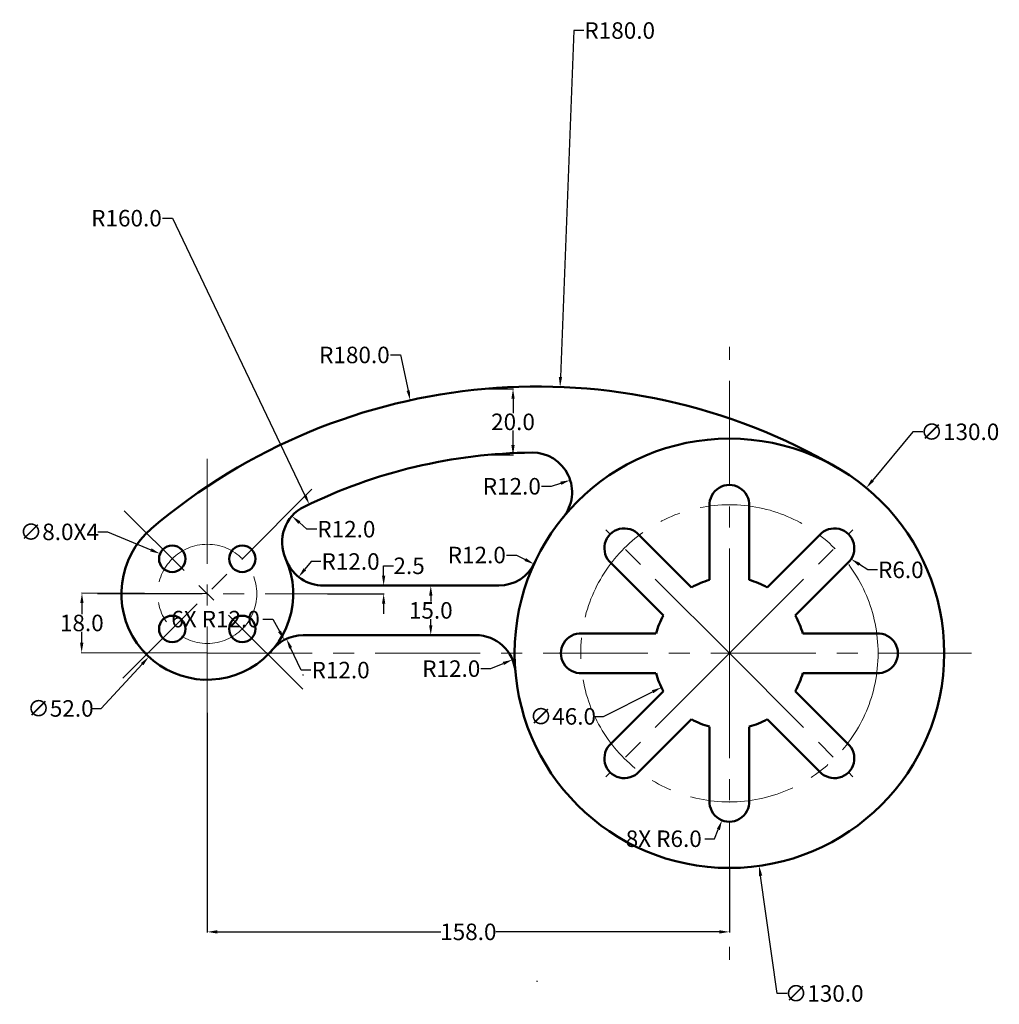
# Model space of a CAD drawing. Units: inches. Extents: x 143 to 440, y 43 to 341.
import ezdxf

# ---------------------------------------------------------------- set-up
doc = ezdxf.new("R2010")
doc.units = ezdxf.units.IN
doc.header["$MEASUREMENT"] = 0
doc.linetypes.add('CENTER', pattern=[50.8, 31.75, -6.35, 6.35, -6.35])
for name, color, linetype, lineweight in [('M-CNTR', 4, 'CENTER', 18), ('M-DIMS', 2, 'Continuous', 25), ('M-OUTL', 7, 'Continuous', 50)]:
    doc.layers.add(name, color=color, linetype=linetype, lineweight=lineweight)
doc.styles.get("Standard").update_dxf_attribs({"font": 'arial.ttf'})
doc.dimstyles.get("Standard").update_dxf_attribs({"dimtxt": 5, "dimasz": 3, "dimexe": 0.18, "dimexo": 0.0625, "dimgap": 0.09, "dimtad": 0, "dimtih": 1, "dimtoh": 1, "dimdec": 1, "dimzin": 0, "dimdsep": 46, "dimtxsty": 'Standard', "dimcen": 0.09, "dimadec": 0, "dimazin": 0, "dimtfac": 1, "dimtdec": 1, "dimtofl": 0, "dimtmove": 0, "dimatfit": 3, "dimfxl": 1, "dimtolj": 1, "dimtzin": 0, "dimarcsym": 0})

# ---------------------------------------------------------------- blocks, each defined once
blk = doc.blocks.new('*D1')
at = {"layer": 'Defpoints', "color": 0, "transparency": 16777216}
for p in [(217.9, 186.39), (182.55, 148.25)]:
    blk.add_point(p, dxfattribs=at)
at = {"layer": 'M-DIMS', "color": 0, "lineweight": -2, "transparency": 16777216}
for p, q in [((200.14, 167.32), (200.32, 167.32)), ((200.23, 167.23), (200.23, 167.41)), ((168.09, 132.63), (180.52, 146.05)), ((165.09, 132.63), (168.09, 132.63))]:
    blk.add_line(p, q, dxfattribs=at)
at = {"layer": 'M-DIMS', "color": 0, "transparency": 16777216}
blk.add_solid([(180.15, 146.39), (180.88, 145.71), (182.55, 148.25)], dxfattribs=at)
at = {"layer": 'M-DIMS', "color": 0, "transparency": 16777216, "insert": (155.79, 132.63), "char_height": 5, "attachment_point": 5}
blk.add_mtext('\\A1;∅52.0', dxfattribs=at)
blk = doc.blocks.new('*D2')
at = {"layer": 'Defpoints', "color": 0, "transparency": 16777216}
for p in [(399.68, 199.38), (316.77, 99.26)]:
    blk.add_point(p, dxfattribs=at)
at = {"layer": 'M-DIMS', "color": 0, "lineweight": -2, "transparency": 16777216}
for p, q in [((413.75, 216.38), (401.59, 201.69)), ((416.75, 216.38), (413.75, 216.38)), ((358.14, 149.32), (358.32, 149.32)), ((358.23, 149.23), (358.23, 149.41))]:
    blk.add_line(p, q, dxfattribs=at)
at = {"layer": 'M-DIMS', "color": 0, "transparency": 16777216}
blk.add_solid([(401.21, 202.01), (401.98, 201.38), (399.68, 199.38)], dxfattribs=at)
at = {"layer": 'M-DIMS', "color": 0, "transparency": 16777216, "insert": (427.99, 216.38), "char_height": 5, "attachment_point": 5}
blk.add_mtext('\\A1;∅130.0', dxfattribs=at)
blk = doc.blocks.new('*D3')
at = {"layer": 'Defpoints', "color": 0, "transparency": 16777216}
for p in [(236.57, 167.32), (243.16, 169.82), (253.6, 169.82)]:
    blk.add_point(p, dxfattribs=at)
at = {"layer": 'M-DIMS', "color": 0, "lineweight": -2, "transparency": 16777216}
for p, q in [((253.6, 172.82), (253.6, 175.82)), ((253.6, 175.82), (256.6, 175.82)), ((236.63, 167.32), (253.78, 167.32)), ((243.22, 169.82), (253.78, 169.82)), ((253.6, 164.32), (253.6, 161.32))]:
    blk.add_line(p, q, dxfattribs=at)
at = {"layer": 'M-DIMS', "color": 0, "transparency": 16777216}
for points in [[(253.1, 172.82), (254.1, 172.82), (253.6, 169.82)], [(253.1, 164.32), (254.1, 164.32), (253.6, 167.32)]]:
    blk.add_solid(points, dxfattribs=at)
at = {"layer": 'M-DIMS', "color": 0, "transparency": 16777216, "insert": (261.3, 175.82), "char_height": 5, "attachment_point": 5}
blk.add_mtext('\\A1;2.5', dxfattribs=at)
blk = doc.blocks.new('*D4')
at = {"layer": 'Defpoints', "color": 0, "transparency": 16777216}
for p in [(267.86, 169.82), (263.59, 154.82), (267.86, 154.82)]:
    blk.add_point(p, dxfattribs=at)
at = {"layer": 'M-DIMS', "color": 0, "lineweight": -2, "transparency": 16777216}
for p, q in [((267.92, 169.82), (268.04, 169.82)), ((267.86, 166.82), (267.86, 164.96)), ((267.86, 157.82), (267.86, 159.68)), ((263.65, 154.82), (268.04, 154.82))]:
    blk.add_line(p, q, dxfattribs=at)
at = {"layer": 'M-DIMS', "color": 0, "transparency": 16777216}
for points in [[(267.36, 166.82), (268.36, 166.82), (267.86, 169.82)], [(267.36, 157.82), (268.36, 157.82), (267.86, 154.82)]]:
    blk.add_solid(points, dxfattribs=at)
at = {"layer": 'M-DIMS', "color": 0, "transparency": 16777216, "insert": (267.86, 162.32), "char_height": 5, "attachment_point": 5}
blk.add_mtext('\\A1;15.0', dxfattribs=at)
blk = doc.blocks.new('*D5')
at = {"layer": 'Defpoints', "color": 0, "transparency": 16777216}
for p in [(261.65, 225.94), (300.09, 50.09)]:
    blk.add_point(p, dxfattribs=at)
at = {"layer": 'M-DIMS', "color": 0, "lineweight": -2, "transparency": 16777216}
for p, q in [((255.66, 239.66), (258.66, 239.66)), ((258.66, 239.66), (261.01, 228.87)), ((300, 50.09), (300.18, 50.09)), ((300.09, 50), (300.09, 50.18))]:
    blk.add_line(p, q, dxfattribs=at)
at = {"layer": 'M-DIMS', "color": 0, "transparency": 16777216}
blk.add_solid([(261.5, 228.98), (260.53, 228.77), (261.65, 225.94)], dxfattribs=at)
at = {"layer": 'M-DIMS', "color": 0, "transparency": 16777216, "insert": (244.75, 239.66), "char_height": 5, "attachment_point": 5}
blk.add_mtext('\\A1;R180.0', dxfattribs=at)
blk = doc.blocks.new('*U6')
blk.add_circle((0, 0), 4)
blk = doc.blocks.new('*U7')
at = {"layer": 'M-OUTL', "color": 0, "linetype": 'ByBlock', "lineweight": -2, "transparency": 16777216}
for p, rotation in [((189.62, 177.93), 89.99999999999999), ((189.62, 156.71), 180), ((210.83, 156.71), 270)]:
    blk.add_blockref('*U6', p, dxfattribs=dict(at, rotation=rotation))
blk.add_blockref('*U6', (210.83, 177.93), dxfattribs=at)
blk = doc.blocks.new('*D8')
at = {"layer": 'Defpoints', "color": 0, "transparency": 16777216}
for p in [(185.93, 179.47), (193.31, 176.39)]:
    blk.add_point(p, dxfattribs=at)
at = {"layer": 'M-DIMS', "color": 0, "lineweight": -2, "transparency": 16777216}
for p, q in [((167.07, 186.09), (170.07, 186.09)), ((170.07, 186.09), (183.16, 180.62)), ((189.53, 177.93), (189.71, 177.93)), ((189.62, 177.84), (189.62, 178.02))]:
    blk.add_line(p, q, dxfattribs=at)
at = {"layer": 'M-DIMS', "color": 0, "transparency": 16777216}
blk.add_solid([(183.35, 181.09), (182.97, 180.16), (185.93, 179.47)], dxfattribs=at)
at = {"layer": 'M-DIMS', "color": 0, "transparency": 16777216, "insert": (155.45, 186.09), "char_height": 5, "attachment_point": 5}
blk.add_mtext('\\A1;∅8.0X4', dxfattribs=at)
blk = doc.blocks.new('*D9')
at = {"layer": 'Defpoints', "color": 0, "transparency": 16777216}
for p in [(224.19, 153.69), (229.27, 142.82)]:
    blk.add_point(p, dxfattribs=at)
at = {"layer": 'M-DIMS', "color": 0, "lineweight": -2, "transparency": 16777216}
for p, q in [((228.61, 144.24), (225.46, 150.97)), ((231.61, 144.24), (228.61, 144.24))]:
    blk.add_line(p, q, dxfattribs=at)
at = {"layer": 'M-DIMS', "color": 0, "transparency": 16777216}
blk.add_solid([(225.91, 151.18), (225, 150.76), (224.19, 153.69)], dxfattribs=at)
at = {"layer": 'M-DIMS', "color": 0, "transparency": 16777216, "insert": (240.58, 144.24), "char_height": 5, "attachment_point": 5}
blk.add_mtext('\\A1;R12.0', dxfattribs=at)
blk = doc.blocks.new('*D10')
at = {"layer": 'Defpoints', "color": 0, "transparency": 16777216}
for p in [(292.6, 147.39), (281.5, 142.82)]:
    blk.add_point(p, dxfattribs=at)
at = {"layer": 'M-DIMS', "color": 0, "lineweight": -2, "transparency": 16777216}
for p, q in [((286.03, 144.68), (289.82, 146.24)), ((283.03, 144.68), (286.03, 144.68))]:
    blk.add_line(p, q, dxfattribs=at)
at = {"layer": 'M-DIMS', "color": 0, "transparency": 16777216}
blk.add_solid([(289.63, 146.71), (290.01, 145.78), (292.6, 147.39)], dxfattribs=at)
at = {"layer": 'M-DIMS', "color": 0, "transparency": 16777216, "insert": (274.06, 144.68), "char_height": 5, "attachment_point": 5}
blk.add_mtext('\\A1;R12.0', dxfattribs=at)
blk = doc.blocks.new('*D11')
at = {"layer": 'Defpoints', "color": 0, "transparency": 16777216}
for p in [(225.85, 190.86), (234.86, 182.94)]:
    blk.add_point(p, dxfattribs=at)
at = {"layer": 'M-DIMS', "color": 0, "lineweight": -2, "transparency": 16777216}
for p, q in [((230.36, 186.9), (228.1, 188.88)), ((233.36, 186.9), (230.36, 186.9))]:
    blk.add_line(p, q, dxfattribs=at)
at = {"layer": 'M-DIMS', "color": 0, "transparency": 16777216}
blk.add_solid([(228.43, 189.26), (227.77, 188.51), (225.85, 190.86)], dxfattribs=at)
at = {"layer": 'M-DIMS', "color": 0, "transparency": 16777216, "insert": (242.32, 186.9), "char_height": 5, "attachment_point": 5}
blk.add_mtext('\\A1;R12.0', dxfattribs=at)
blk = doc.blocks.new('*D12')
at = {"layer": 'Defpoints', "color": 0, "transparency": 16777216}
for p in [(235.35, 181.82), (227.89, 172.42)]:
    blk.add_point(p, dxfattribs=at)
at = {"layer": 'M-DIMS', "color": 0, "lineweight": -2, "transparency": 16777216}
for p, q in [((231.62, 177.12), (229.76, 174.77)), ((234.62, 177.12), (231.62, 177.12))]:
    blk.add_line(p, q, dxfattribs=at)
at = {"layer": 'M-DIMS', "color": 0, "transparency": 16777216}
blk.add_solid([(229.36, 175.08), (230.15, 174.46), (227.89, 172.42)], dxfattribs=at)
at = {"layer": 'M-DIMS', "color": 0, "transparency": 16777216, "insert": (243.59, 177.12), "char_height": 5, "attachment_point": 5}
blk.add_mtext('\\A1;R12.0', dxfattribs=at)
blk = doc.blocks.new('*D13')
at = {"layer": 'Defpoints', "color": 0, "transparency": 16777216}
for p in [(288.42, 181.82), (299.1, 176.34)]:
    blk.add_point(p, dxfattribs=at)
at = {"layer": 'M-DIMS', "color": 0, "lineweight": -2, "transparency": 16777216}
for p, q in [((290.76, 179.08), (293.76, 179.08)), ((293.76, 179.08), (296.43, 177.71))]:
    blk.add_line(p, q, dxfattribs=at)
at = {"layer": 'M-DIMS', "color": 0, "transparency": 16777216}
blk.add_solid([(296.66, 178.16), (296.2, 177.27), (299.1, 176.34)], dxfattribs=at)
at = {"layer": 'M-DIMS', "color": 0, "transparency": 16777216, "insert": (281.79, 179.08), "char_height": 5, "attachment_point": 5}
blk.add_mtext('\\A1;R12.0', dxfattribs=at)
blk = doc.blocks.new('*D14')
at = {"layer": 'Defpoints', "color": 0, "transparency": 16777216}
for p in [(310.07, 201.72), (298.64, 198.09)]:
    blk.add_point(p, dxfattribs=at)
at = {"layer": 'M-DIMS', "color": 0, "lineweight": -2, "transparency": 16777216}
for p, q in [((301.35, 199.9), (304.35, 199.9)), ((304.35, 199.9), (307.21, 200.81))]:
    blk.add_line(p, q, dxfattribs=at)
at = {"layer": 'M-DIMS', "color": 0, "transparency": 16777216}
blk.add_solid([(307.06, 201.29), (307.36, 200.34), (310.07, 201.72)], dxfattribs=at)
at = {"layer": 'M-DIMS', "color": 0, "transparency": 16777216, "insert": (292.39, 199.9), "char_height": 5, "attachment_point": 5}
blk.add_mtext('\\A1;R12.0', dxfattribs=at)
blk = doc.blocks.new('*D15')
at = {"layer": 'Defpoints', "color": 0, "transparency": 16777216}
for p in [(284.3, 229.4), (284.3, 209.4), (292.75, 209.4)]:
    blk.add_point(p, dxfattribs=at)
at = {"layer": 'M-DIMS', "color": 0, "lineweight": -2, "transparency": 16777216}
for p, q in [((284.37, 229.4), (292.93, 229.4)), ((292.75, 226.4), (292.75, 222.04)), ((292.75, 212.4), (292.75, 216.76)), ((284.37, 209.4), (292.93, 209.4))]:
    blk.add_line(p, q, dxfattribs=at)
at = {"layer": 'M-DIMS', "color": 0, "transparency": 16777216}
for points in [[(292.25, 226.4), (293.25, 226.4), (292.75, 229.4)], [(292.25, 212.4), (293.25, 212.4), (292.75, 209.4)]]:
    blk.add_solid(points, dxfattribs=at)
at = {"layer": 'M-DIMS', "color": 0, "transparency": 16777216, "insert": (292.75, 219.4), "char_height": 5, "attachment_point": 5}
blk.add_mtext('\\A1;20.0', dxfattribs=at)
blk = doc.blocks.new('*D16')
at = {"layer": 'Defpoints', "color": 0, "transparency": 16777216}
for p in [(200.32, 167.32), (162.21, 149.51), (200.23, 149.32)]:
    blk.add_point(p, dxfattribs=at)
at = {"layer": 'M-DIMS', "color": 0, "lineweight": -2, "transparency": 16777216}
for p, q in [((200.25, 167.32), (162.12, 167.51)), ((162.28, 164.51), (162.27, 161.15)), ((162.22, 152.51), (162.24, 155.87)), ((200.16, 149.32), (162.03, 149.51))]:
    blk.add_line(p, q, dxfattribs=at)
at = {"layer": 'M-DIMS', "color": 0, "transparency": 16777216}
for points in [[(161.78, 164.51), (162.78, 164.51), (162.3, 167.51)], [(161.72, 152.51), (162.72, 152.51), (162.21, 149.51)]]:
    blk.add_solid(points, dxfattribs=at)
at = {"layer": 'M-DIMS', "color": 0, "transparency": 16777216, "insert": (162.25, 158.51), "char_height": 5, "attachment_point": 5}
blk.add_mtext('\\A1;18.0', dxfattribs=at)
blk = doc.blocks.new('*D17')
at = {"layer": 'Defpoints', "color": 0, "transparency": 16777216}
for p in [(390.04, 181.14), (395.07, 177.87)]:
    blk.add_point(p, dxfattribs=at)
at = {"layer": 'M-DIMS', "color": 0, "lineweight": -2, "transparency": 16777216}
for p, q in [((389.95, 181.14), (390.13, 181.14)), ((390.04, 181.05), (390.04, 181.23)), ((400.1, 174.59), (397.59, 176.23)), ((403.1, 174.59), (400.1, 174.59))]:
    blk.add_line(p, q, dxfattribs=at)
at = {"layer": 'M-DIMS', "color": 0, "transparency": 16777216}
blk.add_solid([(397.86, 176.65), (397.32, 175.81), (395.07, 177.87)], dxfattribs=at)
at = {"layer": 'M-DIMS', "color": 0, "transparency": 16777216, "insert": (410.13, 174.59), "char_height": 5, "attachment_point": 5}
blk.add_mtext('\\A1;R6.0', dxfattribs=at)
blk = doc.blocks.new('*D18')
at = {"layer": 'Defpoints', "color": 0, "transparency": 16777216}
for p in [(378.78, 159.63), (337.67, 139.01)]:
    blk.add_point(p, dxfattribs=at)
at = {"layer": 'M-DIMS', "color": 0, "lineweight": -2, "transparency": 16777216}
for p, q in [((358.14, 149.32), (358.32, 149.32)), ((358.23, 149.23), (358.23, 149.41)), ((320.13, 130.22), (334.98, 137.66)), ((317.13, 130.22), (320.13, 130.22))]:
    blk.add_line(p, q, dxfattribs=at)
at = {"layer": 'M-DIMS', "color": 0, "transparency": 16777216}
blk.add_solid([(334.76, 138.11), (335.21, 137.22), (337.67, 139.01)], dxfattribs=at)
at = {"layer": 'M-DIMS', "color": 0, "transparency": 16777216, "insert": (307.83, 130.22), "char_height": 5, "attachment_point": 5}
blk.add_mtext('\\A1;∅46.0', dxfattribs=at)
blk = doc.blocks.new('*D19')
at = {"layer": 'Defpoints', "color": 0, "transparency": 16777216}
for p in [(200.23, 131.31), (358.23, 84.32), (200.23, 64.98)]:
    blk.add_point(p, dxfattribs=at)
at = {"layer": 'M-DIMS', "color": 0, "lineweight": -2, "transparency": 16777216}
for p, q in [((200.23, 131.25), (200.23, 64.8)), ((358.23, 84.26), (358.23, 64.8)), ((203.23, 64.98), (270.94, 64.98)), ((355.23, 64.98), (287.51, 64.98))]:
    blk.add_line(p, q, dxfattribs=at)
at = {"layer": 'M-DIMS', "color": 0, "transparency": 16777216}
for points in [[(203.23, 65.48), (203.23, 64.48), (200.23, 64.98)], [(355.23, 65.48), (355.23, 64.48), (358.23, 64.98)]]:
    blk.add_solid(points, dxfattribs=at)
at = {"layer": 'M-DIMS', "color": 0, "transparency": 16777216, "insert": (279.23, 64.98), "char_height": 5, "attachment_point": 5}
blk.add_mtext('\\A1;158.0', dxfattribs=at)
blk = doc.blocks.new('*D20')
at = {"layer": 'Defpoints', "color": 0, "transparency": 16777216}
for p in [(307, 229.96), (300.09, 50.09)]:
    blk.add_point(p, dxfattribs=at)
at = {"layer": 'M-DIMS', "color": 0, "lineweight": -2, "transparency": 16777216}
for p, q in [((311.14, 337.88), (307.11, 232.96)), ((314.14, 337.88), (311.14, 337.88)), ((300, 50.09), (300.18, 50.09)), ((300.09, 50), (300.09, 50.18))]:
    blk.add_line(p, q, dxfattribs=at)
at = {"layer": 'M-DIMS', "color": 0, "transparency": 16777216}
blk.add_solid([(306.61, 232.98), (307.61, 232.94), (307, 229.96)], dxfattribs=at)
at = {"layer": 'M-DIMS', "color": 0, "transparency": 16777216, "insert": (325.05, 337.88), "char_height": 5, "attachment_point": 5}
blk.add_mtext('\\A1;R180.0', dxfattribs=at)
blk = doc.blocks.new('*D21')
at = {"layer": 'Defpoints', "color": 0, "transparency": 16777216}
for p in [(231.09, 194.45), (300.09, 50.09)]:
    blk.add_point(p, dxfattribs=at)
at = {"layer": 'M-DIMS', "color": 0, "lineweight": -2, "transparency": 16777216}
for p, q in [((186.68, 281.06), (189.68, 281.06)), ((189.68, 281.06), (229.79, 197.15)), ((300, 50.09), (300.18, 50.09)), ((300.09, 50), (300.09, 50.18))]:
    blk.add_line(p, q, dxfattribs=at)
at = {"layer": 'M-DIMS', "color": 0, "transparency": 16777216}
blk.add_solid([(230.24, 197.37), (229.34, 196.94), (231.09, 194.45)], dxfattribs=at)
at = {"layer": 'M-DIMS', "color": 0, "transparency": 16777216, "insert": (175.77, 281.06), "char_height": 5, "attachment_point": 5}
blk.add_mtext('\\A1;R160.0', dxfattribs=at)
blk = doc.blocks.new('*D22')
at = {"layer": 'Defpoints', "color": 0, "transparency": 16777216}
for p in [(223.53, 153.36), (229.27, 142.82)]:
    blk.add_point(p, dxfattribs=at)
at = {"layer": 'M-DIMS', "color": 0, "lineweight": -2, "transparency": 16777216}
for p, q in [((217.08, 159.68), (220.08, 159.68)), ((220.08, 159.68), (222.09, 155.99)), ((229.18, 142.82), (229.36, 142.82)), ((229.27, 142.73), (229.27, 142.91))]:
    blk.add_line(p, q, dxfattribs=at)
at = {"layer": 'M-DIMS', "color": 0, "transparency": 16777216}
blk.add_solid([(222.53, 156.23), (221.65, 155.75), (223.53, 153.36)], dxfattribs=at)
at = {"layer": 'M-DIMS', "color": 0, "transparency": 16777216, "insert": (202.73, 159.68), "char_height": 5, "attachment_point": 5}
blk.add_mtext('\\A1;6X R12.0', dxfattribs=at)
blk = doc.blocks.new('*D23')
at = {"layer": 'Defpoints', "color": 0, "transparency": 16777216}
for p in [(349.19, 213.69), (367.26, 84.95)]:
    blk.add_point(p, dxfattribs=at)
at = {"layer": 'M-DIMS', "color": 0, "lineweight": -2, "transparency": 16777216}
for p, q in [((358.14, 149.32), (358.32, 149.32)), ((358.23, 149.23), (358.23, 149.41)), ((372.68, 46.33), (367.68, 81.98)), ((375.68, 46.33), (372.68, 46.33))]:
    blk.add_line(p, q, dxfattribs=at)
at = {"layer": 'M-DIMS', "color": 0, "transparency": 16777216}
blk.add_solid([(368.17, 82.05), (367.18, 81.91), (367.26, 84.95)], dxfattribs=at)
at = {"layer": 'M-DIMS', "color": 0, "transparency": 16777216, "insert": (386.92, 46.33), "char_height": 5, "attachment_point": 5}
blk.add_mtext('\\A1;∅130.0', dxfattribs=at)
blk = doc.blocks.new('*D24')
at = {"layer": 'Defpoints', "color": 0, "transparency": 16777216}
for p in [(358.23, 104.32), (356, 98.75)]:
    blk.add_point(p, dxfattribs=at)
at = {"layer": 'M-DIMS', "color": 0, "lineweight": -2, "transparency": 16777216}
for p, q in [((358.23, 104.23), (358.23, 104.41)), ((358.14, 104.32), (358.32, 104.32)), ((353.77, 93.18), (354.89, 95.96)), ((350.77, 93.18), (353.77, 93.18))]:
    blk.add_line(p, q, dxfattribs=at)
at = {"layer": 'M-DIMS', "color": 0, "transparency": 16777216}
blk.add_solid([(354.42, 96.15), (355.35, 95.78), (356, 98.75)], dxfattribs=at)
at = {"layer": 'M-DIMS', "color": 0, "transparency": 16777216, "insert": (338.37, 93.18), "char_height": 5, "attachment_point": 5}
blk.add_mtext('\\A1;8X R6.0', dxfattribs=at)

msp = doc.modelspace()

# ---------------------------------------------------------------- linework, layer by layer
at = {"layer": 'M-CNTR'}
for p, q in [((358.23, 149.32), (358.23, 242.13)), ((200.23, 208.21), (200.23, 131.31)), ((174.71, 141.81), (231.88, 198.98)), ((229.1, 138.44), (175.11, 192.44)), ((358.23, 149.32), (320.88, 186.67)), ((358.23, 149.32), (395.57, 186.67)), ((166.96, 167.32), (237.3, 167.32)), ((200.23, 149.32), (431.53, 149.32)), ((358.23, 149.32), (320.88, 111.97)), ((358.23, 149.32), (358.23, 56.51)), ((358.23, 149.32), (395.57, 111.97))]:
    msp.add_line(p, q, dxfattribs=at)
for centre, radius in [((358.23, 149.32), 45), ((200.23, 167.32), 15)]:
    msp.add_circle(centre, radius, dxfattribs=at)
at = {"layer": 'M-OUTL'}
for p, q in [((352.24, 193.92), (352.24, 171.53)), ((364.21, 193.92), (364.21, 171.53)), ((346.77, 169.26), (330.65, 185.38)), ((369.68, 169.26), (385.8, 185.38)), ((338.28, 160.78), (322.16, 176.9)), ((378.17, 160.78), (394.29, 176.9)), ((235.35, 169.82), (288.42, 169.82)), ((336.02, 155.32), (313.23, 155.32)), ((380.43, 155.32), (403.23, 155.32)), ((229.27, 154.82), (281.5, 154.82)), ((336.02, 143.32), (313.23, 143.32)), ((380.43, 143.32), (403.23, 143.32)), ((338.28, 137.86), (322.16, 121.74)), ((378.17, 137.86), (394.29, 121.74)), ((346.77, 129.38), (330.65, 113.26)), ((369.68, 129.38), (385.8, 113.26)), ((352.24, 104.72), (352.24, 127.11)), ((364.21, 104.72), (364.21, 127.11))]:
    msp.add_line(p, q, dxfattribs=at)
msp.add_circle((358.23, 149.32), 65, dxfattribs=at)
for centre, radius, start, end in [((300.09, 50.09), 180, 59.6368, 130.429), ((300.09, 50.09), 160, 90.5647, 116.1513), ((298.64, 198.09), 12, 320.7038, 90.5647), ((358.23, 194.32), 6, 356.1774, 183.8226), ((234.86, 182.94), 12, 116.1513, 204.2764), ((200.23, 167.32), 26, 130.429, 24.2764), ((326.41, 181.14), 6, 41.1774, 228.8226), ((390.04, 181.14), 6, 311.1774, 138.8226), ((235.35, 181.82), 12, 202.4315, 270), ((288.42, 181.82), 12, 270, 335.0342), ((358.23, 149.32), 23, 105.0872, 119.8783), ((358.23, 149.32), 23, 60.1217, 74.9128), ((358.23, 149.32), 23, 150.1217, 164.8783), ((358.23, 149.32), 23, 15.1217, 29.8783), ((313.23, 149.32), 6, 86.1774, 273.8226), ((403.23, 149.32), 6, 266.1774, 93.8226), ((229.27, 142.82), 12, 90, 147.2028), ((281.5, 142.82), 12, 4.8424, 90), ((358.23, 149.32), 23, 195.1217, 209.8783), ((358.23, 149.32), 23, 330.1217, 344.8783), ((358.23, 149.32), 23, 240.1217, 254.9128), ((358.23, 149.32), 23, 285.0872, 299.8783), ((326.41, 117.5), 6, 131.1774, 318.8226), ((390.04, 117.5), 6, 221.1774, 48.8226), ((358.23, 104.32), 6, 176.1774, 3.8226)]:
    msp.add_arc(centre, radius, start, end, dxfattribs=at)

# ---------------------------------------------------------------- block references
msp.add_blockref('*U7', (0, 0), dxfattribs=at)

# ---------------------------------------------------------------- dimensions: what is measured, and where the dimension line sits
at = {"layer": 'M-DIMS'}
for center, mpoint, override, picture, middle in [((300.09, 50.09), (307, 229.96), {"dimdec": 1, "dimlfac": 1, "dimrnd": 0, "dimzin": 0, "dimdsep": 46, "dimlunit": 2}, '*D20', (325.05, 337.88)), ((300.09, 50.09), (231.09, 194.45), {"dimdec": 1, "dimlfac": 1, "dimrnd": 0, "dimzin": 0, "dimdsep": 46, "dimlunit": 2}, '*D21', (175.77, 281.06)), ((300.09, 50.09), (261.65, 225.94), {"dimclrd": 0, "dimclre": 0, "dimclrt": 0}, '*D5', (244.75, 239.66)), ((298.64, 198.09), (310.07, 201.72), {"dimclrd": 0, "dimclre": 0, "dimclrt": 0}, '*D14', (292.39, 199.9)), ((234.86, 182.94), (225.85, 190.86), {"dimclrd": 0, "dimclre": 0, "dimclrt": 0}, '*D11', (242.32, 186.9)), ((288.42, 181.82), (299.1, 176.34), {"dimclrd": 0, "dimclre": 0, "dimclrt": 0}, '*D13', (281.79, 179.08)), ((235.35, 181.82), (227.89, 172.42), {"dimclrd": 0, "dimclre": 0, "dimclrt": 0}, '*D12', (243.59, 177.12)), ((229.27, 142.82), (224.19, 153.69), {"dimclrd": 0, "dimclre": 0, "dimclrt": 0}, '*D9', (240.58, 144.24)), ((281.5, 142.82), (292.6, 147.39), {"dimclrd": 0, "dimclre": 0, "dimclrt": 0}, '*D10', (274.06, 144.68))]:
    dim = msp.add_radius_dim(center=center, mpoint=mpoint, dimstyle='Standard', override=override, dxfattribs=at)
    dim.commit()
    dim.dimension.update_dxf_attribs({"geometry": picture, "text_midpoint": middle, "dimtype": 164})
for base, p1, p2, picture, middle in [((292.75, 209.4), (284.3, 229.4), (284.3, 209.4), '*D15', (292.75, 219.4)), ((267.86, 154.82), (267.86, 169.82), (263.59, 154.82), '*D4', (267.86, 162.32))]:
    dim = msp.add_linear_dim(base=base, p1=p1, p2=p2, angle=90, dimstyle='Standard', override={"dimclrd": 0, "dimclre": 0, "dimclrt": 0}, dxfattribs=at)
    dim.commit()
    dim.dimension.update_dxf_attribs({"geometry": picture, "text_midpoint": middle})
for p1, p2, override, picture, middle in [((316.77, 99.26), (399.68, 199.38), {"dimclrd": 0, "dimclre": 0, "dimclrt": 0}, '*D2', (427.99, 216.38)), ((349.19, 213.69), (367.26, 84.95), {"dimdec": 1, "dimlfac": 1, "dimrnd": 0, "dimzin": 0, "dimdsep": 46, "dimlunit": 2}, '*D23', (386.92, 46.33)), ((217.9, 186.39), (182.55, 148.25), {"dimclrd": 0, "dimclre": 0, "dimclrt": 0}, '*D1', (155.79, 132.63)), ((378.78, 159.63), (337.67, 139.01), {"dimclrd": 0, "dimclre": 0, "dimclrt": 0}, '*D18', (307.83, 130.22))]:
    dim = msp.add_diameter_dim_2p(p1=p1, p2=p2, dimstyle='Standard', override=override, dxfattribs=at)
    dim.commit()
    dim.dimension.update_dxf_attribs({"geometry": picture, "text_midpoint": middle, "dimtype": 163})
dim = msp.add_diameter_dim_2p(p1=(193.31, 176.39), p2=(185.93, 179.47), text='<>X4', dimstyle='Standard', override={"dimclrd": 0, "dimclre": 0, "dimclrt": 0}, dxfattribs=at)
dim.commit()
dim.dimension.update_dxf_attribs({"geometry": '*D8', "text_midpoint": (155.45, 186.09), "dimtype": 163})
dim = msp.add_linear_dim(base=(253.6, 169.82), p1=(236.57, 167.32), p2=(243.16, 169.82), angle=90, dimstyle='Standard', override={"dimclrd": 0, "dimclre": 0, "dimclrt": 0}, dxfattribs=at)
dim.commit()
dim.dimension.update_dxf_attribs({"geometry": '*D3', "text_midpoint": (261.3, 175.82), "dimtype": 160})
dim = msp.add_radius_dim(center=(390.04, 181.14), mpoint=(395.07, 177.87), dimstyle='Standard', override={"dimclrd": 0, "dimclre": 0, "dimclrt": 0}, dxfattribs=at)
dim.commit()
dim.dimension.update_dxf_attribs({"geometry": '*D17', "text_midpoint": (410.13, 174.59)})
dim = msp.add_aligned_dim(p1=(200.32, 167.32), p2=(200.23, 149.32), distance=-38.02, dimstyle='Standard', override={"dimclrd": 0, "dimclre": 0, "dimclrt": 0}, dxfattribs=at)
dim.commit()
dim.dimension.update_dxf_attribs({"geometry": '*D16', "text_midpoint": (162.25, 158.51)})
dim = msp.add_radius_dim(center=(229.27, 142.82), mpoint=(223.53, 153.36), text='6X <>', dimstyle='Standard', override={"dimdec": 1, "dimlfac": 1, "dimrnd": 0, "dimzin": 0, "dimdsep": 46, "dimlunit": 2}, dxfattribs=at)
dim.commit()
dim.dimension.update_dxf_attribs({"geometry": '*D22', "text_midpoint": (202.73, 159.68), "dimtype": 164})
dim = msp.add_linear_dim(base=(200.23, 64.98), p1=(358.23, 84.32), p2=(200.23, 131.31), dimstyle='Standard', override={"dimclrd": 0, "dimclre": 0, "dimclrt": 0}, dxfattribs=at)
dim.commit()
dim.dimension.update_dxf_attribs({"geometry": '*D19', "text_midpoint": (279.23, 64.98)})
dim = msp.add_radius_dim(center=(358.23, 104.32), mpoint=(356, 98.75), text='8X <>', dimstyle='Standard', override={"dimdec": 1, "dimlfac": 1, "dimrnd": 0, "dimzin": 0, "dimdsep": 46, "dimlunit": 2}, dxfattribs=at)
dim.commit()
dim.dimension.update_dxf_attribs({"geometry": '*D24', "text_midpoint": (338.37, 93.18)})

doc.saveas('drawing.dxf')
